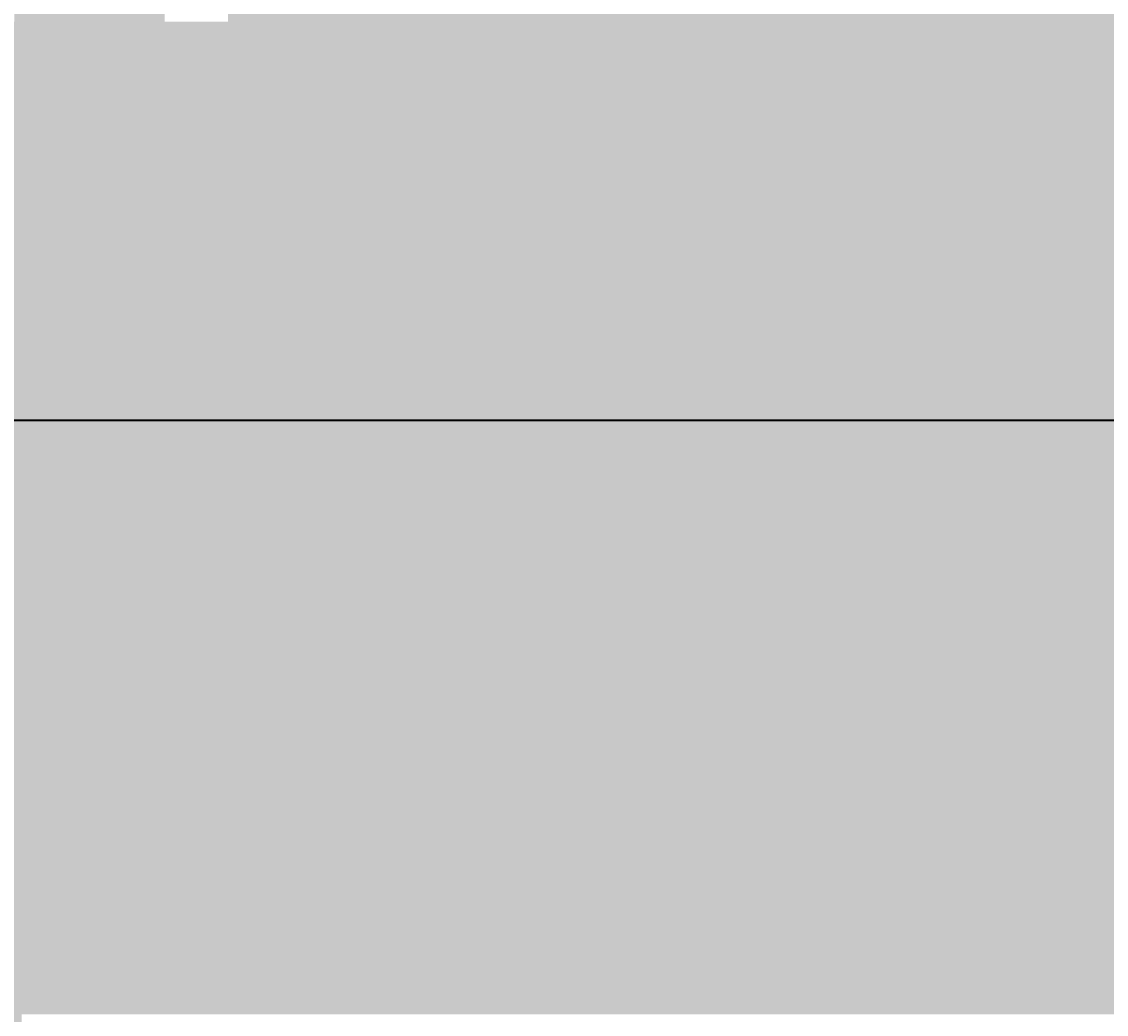
# Model space of a CAD drawing. Units: feet. Extents: x 2695 to 2912, y 795 to 1139.
# Tile 28 of 83: x 2774 to 2808, y 906 to 937. Entities that reach past the tile are written whole.
import ezdxf

# ---------------------------------------------------------------- set-up
doc = ezdxf.new("R2010")
doc.units = ezdxf.units.FT
for name, color, linetype, lineweight in [('A-ANNO-DIMS', 2, 'Continuous', 18), ('A-ELEV', 7, 'Continuous', 35), ('A-ELEV-PATT', 252, 'Continuous', 13)]:
    doc.layers.add(name, color=color, linetype=linetype, lineweight=lineweight)
doc.styles.get("Standard").update_dxf_attribs({"font": 'arial.ttf'})
doc.dimstyles.get("Standard").update_dxf_attribs({"dimtxt": 0.18, "dimasz": 0.18, "dimexe": 0.18, "dimexo": 0.0625, "dimgap": 0.09, "dimtad": 0, "dimtih": 1, "dimtoh": 1, "dimdec": 1, "dimzin": 0, "dimdsep": 46, "dimlunit": 3, "dimtxsty": 'Standard', "dimcen": 0.09, "dimadec": 0, "dimazin": 0, "dimtfac": 1, "dimtdec": 1, "dimtofl": 0, "dimtmove": 0, "dimatfit": 3, "dimfxl": 1, "dimtolj": 1, "dimtzin": 0, "dimarcsym": 0})

# ---------------------------------------------------------------- blocks, each defined once
blk = doc.blocks.new('*D14')
at = {"layer": 'A-ANNO-DIMS', "color": 0, "lineweight": -2, "transparency": 16777216}
for p, q in [((2838.439, 905.514), (2911.424, 905.514)), ((2911.244, 905.334), (2911.244, 890.368)), ((2911.244, 875.037), (2911.244, 890.004)), ((2758.214, 874.857), (2911.424, 874.857))]:
    blk.add_line(p, q, dxfattribs=at)
at = {"layer": 'A-ANNO-DIMS', "color": 0, "transparency": 16777216}
for points in [[(2911.214, 905.334), (2911.274, 905.334), (2911.244, 905.514)], [(2911.214, 875.037), (2911.274, 875.037), (2911.244, 874.857)]]:
    blk.add_solid(points, dxfattribs=at)
at = {"layer": 'Defpoints', "color": 0, "transparency": 16777216}
for p in [(2838.377, 905.514), (2911.244, 905.514), (2758.151, 874.857)]:
    blk.add_point(p, dxfattribs=at)
at = {"layer": 'A-ANNO-DIMS', "color": 0, "transparency": 16777216, "insert": (2911.244, 890.186), "char_height": 0.18, "attachment_point": 5}
blk.add_mtext('\\A1;30.66', dxfattribs=at)

msp = doc.modelspace()

# ---------------------------------------------------------------- hatches: boundary and pattern name
at = {"layer": 'A-ELEV-PATT'}
h = msp.add_hatch(color=256, dxfattribs=at)
h.set_gradient(color1=(255, 255, 255), tint=1)
h.paths.add_polyline_path([(2770.6361, 1122.9306), (2710.6361, 1122.9306), (2710.6361, 1118.4096), (2770.6361, 1118.4096)])
h.paths.add_polyline_path([(2890.6361, 1107.8588), (2770.6361, 1107.8588), (2770.6361, 1103.3378), (2890.6361, 1103.3378)])
h.paths.add_polyline_path([(2890.6361, 1062.9306), (2710.6361, 1062.9306), (2710.6361, 1056.9306), (2710.6361, 936.9306), (2710.6361, 924.3105), (2716.5358, 924.3105), (2890.6361, 924.3105), (2890.6361, 936.9306), (2715.8852, 936.9306), (2715.8852, 1050.3105), (2890.6361, 1050.3105)])
h.paths.add_polyline_path([(2716.5358, 924.3105), (2710.6361, 924.3105), (2710.6361, 810.9306), (2716.5358, 810.9306)])
h = msp.add_hatch(color=256, dxfattribs=at)
h.set_gradient(color1=(147, 149, 152), color2=(147, 149, 152), tint=1)
h.paths.add_polyline_path([(2770.6361, 1118.4096), (2710.6361, 1118.4096), (2710.6361, 1062.9306), (2770.6361, 1062.9306)])
h.paths.add_polyline_path([(2890.6361, 1103.3378), (2770.6361, 1103.3378), (2770.6361, 1062.9306), (2890.6361, 1062.9306)])
h.paths.add_polyline_path([(2730.7081, 1048.1052), (2755.1125, 1048.1052), (2755.1125, 936.9306), (2770.6361, 936.9306), (2770.6361, 1050.3105), (2715.8852, 1050.3105), (2715.8852, 936.9306), (2730.7081, 936.9306)])
h.paths.add_polyline_path([(2890.6361, 1050.3105), (2770.6361, 1050.3105), (2770.6361, 971.9673), (2778.0341, 971.9673), (2778.0341, 1020.8235), (2843.575, 1020.8235), (2843.575, 971.9673), (2890.6361, 971.9673)])
h.paths.add_polyline_path([(2888.1882, 970.7156), (2843.575, 970.7156), (2843.575, 964.8267), (2888.1882, 964.8267)])
h.paths.add_polyline_path([(2888.1882, 964.1328), (2843.575, 964.1328), (2843.575, 956.614), (2888.1882, 956.614)])
h.paths.add_polyline_path([(2888.1882, 955.9202), (2843.575, 955.9202), (2843.575, 949.2892), (2888.1882, 949.2892)])
h.paths.add_polyline_path([(2888.1882, 948.5954), (2843.575, 948.5954), (2843.575, 941.3507), (2888.1882, 941.3507)])
h.paths.add_polyline_path([(2888.1882, 940.6569), (2843.575, 940.6569), (2843.575, 936.9306), (2888.1882, 936.9306)])
h.paths.add_polyline_path([(2890.6361, 970.7156), (2888.9368, 970.7156), (2888.9368, 964.8267), (2890.6361, 964.8267)])
h.paths.add_polyline_path([(2890.6361, 964.1328), (2888.9368, 964.1328), (2888.9368, 956.614), (2890.6361, 956.614)])
h.paths.add_polyline_path([(2890.6361, 955.9202), (2888.9368, 955.9202), (2888.9368, 949.2892), (2890.6361, 949.2892)])
h.paths.add_polyline_path([(2890.6361, 940.6569), (2888.9368, 940.6569), (2888.9368, 936.9306), (2890.6361, 936.9306)])
h.paths.add_polyline_path([(2890.6361, 948.5954), (2888.9368, 948.5954), (2888.9368, 941.3507), (2890.6361, 941.3507)])
h.paths.add_polyline_path([(2772.5216, 970.7156), (2770.6361, 970.7156), (2770.6361, 964.8267), (2772.5216, 964.8267)])
h.paths.add_polyline_path([(2772.5216, 964.1328), (2770.6361, 964.1328), (2770.6361, 956.614), (2772.5216, 956.614)])
h.paths.add_polyline_path([(2772.5216, 955.9202), (2770.6361, 955.9202), (2770.6361, 949.2892), (2772.5216, 949.2892)])
h.paths.add_polyline_path([(2772.5216, 948.5954), (2770.6361, 948.5954), (2770.6361, 941.3507), (2772.5216, 941.3507)])
h.paths.add_polyline_path([(2772.5216, 940.6569), (2770.6361, 940.6569), (2770.6361, 936.9306), (2772.5216, 936.9306)])
h.paths.add_polyline_path([(2778.0341, 940.6569), (2773.2702, 940.6569), (2773.2702, 936.9306), (2778.0341, 936.9306)])
h.paths.add_polyline_path([(2778.0341, 970.7156), (2773.2702, 970.7156), (2773.2702, 964.8267), (2778.0341, 964.8267)])
h.paths.add_polyline_path([(2778.0341, 964.1328), (2773.2702, 964.1328), (2773.2702, 956.614), (2778.0341, 956.614)])
h.paths.add_polyline_path([(2778.0341, 955.9202), (2773.2702, 955.9202), (2773.2702, 949.2892), (2778.0341, 949.2892)])
h.paths.add_polyline_path([(2778.0341, 948.5954), (2773.2702, 948.5954), (2773.2702, 941.3507), (2778.0341, 941.3507)])
h.paths.add_polyline_path([(2810.0407, 940.6569), (2780.0341, 940.6569), (2780.0341, 936.9306), (2810.0407, 936.9306)])
h.paths.add_polyline_path([(2890.6361, 924.3105), (2770.6361, 924.3105), (2770.6361, 810.9306), (2773.5029, 810.9306), (2773.5029, 905.5143), (2805.9398, 905.5143), (2838.3767, 905.5143), (2838.3767, 810.9306), (2890.6361, 810.9306)])

# ---------------------------------------------------------------- linework, layer by layer
at = {"layer": 'A-ELEV'}
msp.add_lwpolyline([(2890.6361, 936.9306), (2890.6361, 924.3105), (2710.6361, 924.3105), (2710.6361, 936.9306)], dxfattribs=at)

# ---------------------------------------------------------------- dimensions: what is measured, and where the dimension line sits
at = {"layer": 'A-ANNO-DIMS'}
dim = msp.add_linear_dim(base=(2911.2444, 905.5143), p1=(2758.1515, 874.8571), p2=(2838.3767, 905.5143), angle=90, dimstyle='Standard', override={"dimdec": 2, "dimlfac": 1, "dimrnd": 0, "dimzin": 0, "dimdsep": 46, "dimlunit": 2}, dxfattribs=at)
dim.commit()
dim.dimension.update_dxf_attribs({"geometry": '*D14', "text_midpoint": (2911.2444, 890.1857)})

doc.saveas('drawing.dxf')
